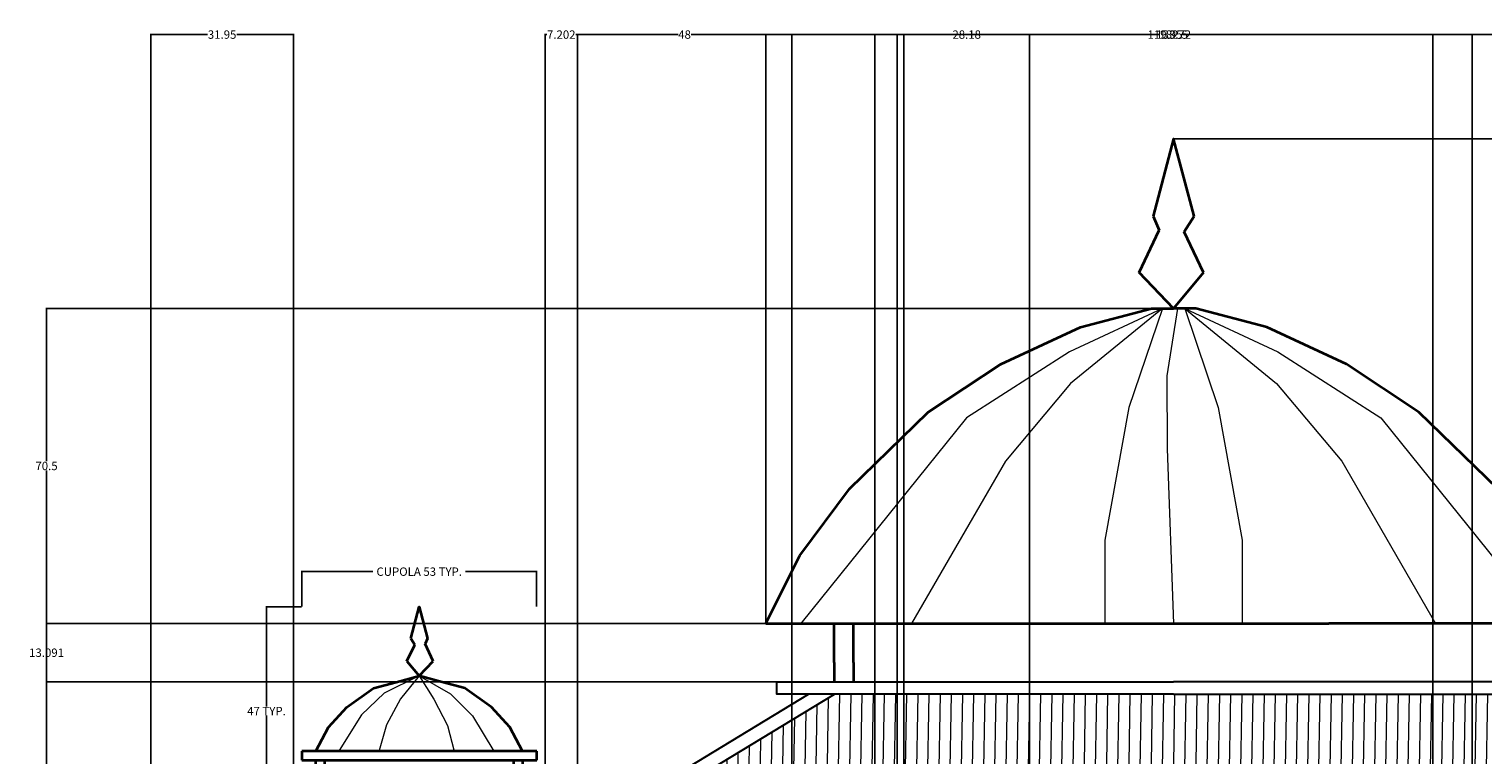
# Model space of a CAD drawing. Units: inches. Extents: x 4 to 523, y 84 to 443.
# Tile 2 of 3: x 4 to 329, y 281 to 443. Entities that reach past the tile are written whole.
import ezdxf

# ---------------------------------------------------------------- set-up
doc = ezdxf.new("R2010")
doc.units = ezdxf.units.IN
doc.header["$MEASUREMENT"] = 0
for name, color, linetype, lineweight in [('A-ANNO-DIMS', 2, 'Continuous', 18), ('A-ROOF', 7, 'Continuous', 30), ('A-ROOF-DETL', 3, 'Continuous', 18), ('A-ROOF-DOME', 7, 'Continuous', 35), ('A-ROOF-PATT', 252, 'Continuous', 13)]:
    doc.layers.add(name, color=color, linetype=linetype, lineweight=lineweight)
doc.styles.get("Standard").update_dxf_attribs({"font": 'arial.ttf'})
doc.dimstyles.get("Standard").update_dxf_attribs({"dimtxt": 1.875, "dimasz": 0.18, "dimexe": 0.18, "dimexo": 0.0625, "dimgap": 0.09, "dimtad": 0, "dimtih": 1, "dimtoh": 1, "dimdec": 4, "dimzin": 0, "dimdsep": 46, "dimlunit": 4, "dimtxsty": 'Standard', "dimcen": 0.09, "dimadec": 0, "dimazin": 0, "dimtfac": 1, "dimtdec": 4, "dimtofl": 0, "dimtmove": 0, "dimatfit": 3, "dimfxl": 1, "dimtolj": 1, "dimtzin": 0, "dimarcsym": 0})

# ---------------------------------------------------------------- blocks, each defined once
blk = doc.blocks.new('CUPOLA-PROFILE')
for p, q in [((52.59, 14.33), (0, 14.33)), ((0, 14.33), (0, 12.33)), ((52.59, 12.33), (52.59, 14.33)), ((0, 12.33), (52.59, 12.33)), ((3.17, 3.77), (3.17, 12.33)), ((5.17, 3.77), (5.17, 12.33)), ((47.49, 3.77), (47.49, 12.33)), ((49.49, 3.77), (49.49, 12.33)), ((3.17, 3.77), (3.17, 0)), ((5.17, 3.77), (5.17, 0)), ((47.49, 3.77), (47.49, 0)), ((49.49, 3.77), (49.49, 0))]:
    blk.add_line(p, q)
for points in [[(24.44, 39.59), (26.29, 46.64), (28.15, 39.59)], [(25.33, 38.18), (24.44, 39.59)], [(28.15, 39.59), (27.62, 38.34)], [(23.56, 34.47), (25.33, 38.18)], [(29.42, 34.47), (27.62, 38.34)], [(23.56, 34.47), (26.29, 31.2)], [(26.29, 31.2), (29.42, 34.47)], [(3.17, 14.33), (6, 19.75), (10.13, 24.22), (16.05, 28.42), (21.12, 29.8), (26.29, 31.2)], [(49.42, 14.33), (46.59, 19.75), (42.46, 24.22), (36.53, 28.42), (31.46, 29.8), (26.29, 31.2)]]:
    blk.add_lwpolyline(points)
blk = doc.blocks.new('*D11')
at = {"layer": 'A-ANNO-DIMS', "color": 0, "lineweight": -2, "transparency": 16777216}
for p, q in [((64.71, 313.84), (64.71, 321.84)), ((64.89, 321.66), (80.62, 321.66)), ((117.12, 321.66), (101.4, 321.66)), ((117.3, 313.84), (117.3, 321.84))]:
    blk.add_line(p, q, dxfattribs=at)
at = {"layer": 'A-ANNO-DIMS', "color": 0, "transparency": 16777216}
for points in [[(64.89, 321.69), (64.89, 321.63), (64.71, 321.66)], [(117.12, 321.69), (117.12, 321.63), (117.3, 321.66)]]:
    blk.add_solid(points, dxfattribs=at)
at = {"layer": 'Defpoints', "color": 0, "transparency": 16777216}
for p in [(117.3, 321.66), (64.71, 313.78), (117.3, 313.78)]:
    blk.add_point(p, dxfattribs=at)
at = {"layer": 'A-ANNO-DIMS', "color": 0, "transparency": 16777216, "insert": (91.01, 321.66), "char_height": 1.875, "attachment_point": 5}
blk.add_mtext('\\A1;CUPOLA 53 TYP.', dxfattribs=at)
blk = doc.blocks.new('*D12')
at = {"layer": 'A-ANNO-DIMS', "color": 0, "lineweight": -2, "transparency": 16777216}
for p, q in [((64.65, 313.78), (56.65, 313.78)), ((56.83, 313.6), (56.83, 291.48)), ((56.83, 267.31), (56.83, 289.43)), ((64.65, 267.13), (56.65, 267.13))]:
    blk.add_line(p, q, dxfattribs=at)
at = {"layer": 'A-ANNO-DIMS', "color": 0, "transparency": 16777216}
for points in [[(56.8, 313.6), (56.86, 313.6), (56.83, 313.78)], [(56.8, 267.31), (56.86, 267.31), (56.83, 267.13)]]:
    blk.add_solid(points, dxfattribs=at)
at = {"layer": 'Defpoints', "color": 0, "transparency": 16777216}
for p in [(56.83, 313.78), (64.71, 313.78), (64.71, 267.13)]:
    blk.add_point(p, dxfattribs=at)
at = {"layer": 'A-ANNO-DIMS', "color": 0, "transparency": 16777216, "insert": (56.83, 290.45), "char_height": 1.875, "attachment_point": 5}
blk.add_mtext('\\A1;47 TYP.', dxfattribs=at)
blk = doc.blocks.new('*D20')
at = {"layer": 'A-ANNO-DIMS', "color": 0, "lineweight": -2, "transparency": 16777216}
for p, q in [((259.93, 418.56), (519, 418.56)), ((518.82, 418.38), (518.82, 265.56)), ((518.82, 110.64), (518.82, 263.46)), ((495.56, 110.46), (519, 110.46))]:
    blk.add_line(p, q, dxfattribs=at)
at = {"layer": 'A-ANNO-DIMS', "color": 0, "transparency": 16777216}
for points in [[(518.79, 418.38), (518.85, 418.38), (518.82, 418.56)], [(518.79, 110.64), (518.85, 110.64), (518.82, 110.46)]]:
    blk.add_solid(points, dxfattribs=at)
at = {"layer": 'Defpoints', "color": 0, "transparency": 16777216}
for p in [(259.87, 418.56), (518.82, 418.56), (495.5, 110.46)]:
    blk.add_point(p, dxfattribs=at)
at = {"layer": 'A-ANNO-DIMS', "color": 0, "transparency": 16777216, "insert": (518.82, 264.51), "char_height": 1.875, "attachment_point": 5}
blk.add_mtext('\\A1;308.1', dxfattribs=at)
blk = doc.blocks.new('*D21')
at = {"layer": 'A-ANNO-DIMS', "color": 0, "lineweight": -2, "transparency": 16777216}
for p, q in [((30.92, 119.64), (30.92, 442.06)), ((31.1, 441.88), (43.64, 441.88)), ((62.69, 441.88), (50.16, 441.88)), ((62.87, 128.52), (62.87, 442.06))]:
    blk.add_line(p, q, dxfattribs=at)
at = {"layer": 'A-ANNO-DIMS', "color": 0, "transparency": 16777216}
for points in [[(31.1, 441.91), (31.1, 441.85), (30.92, 441.88)], [(62.69, 441.91), (62.69, 441.85), (62.87, 441.88)]]:
    blk.add_solid(points, dxfattribs=at)
at = {"layer": 'Defpoints', "color": 0, "transparency": 16777216}
for p in [(62.87, 441.88), (62.87, 128.46), (30.92, 119.58)]:
    blk.add_point(p, dxfattribs=at)
at = {"layer": 'A-ANNO-DIMS', "color": 0, "transparency": 16777216, "insert": (46.9, 441.88), "char_height": 1.875, "attachment_point": 5}
blk.add_mtext('\\A1;31.95', dxfattribs=at)
blk = doc.blocks.new('*D24')
at = {"layer": 'A-ANNO-DIMS', "color": 0, "lineweight": -2, "transparency": 16777216}
for p, q in [((168.55, 310.07), (7.42, 310.07)), ((7.6, 309.89), (7.6, 220.31)), ((7.6, 128.64), (7.6, 218.22)), ((47.09, 128.46), (7.42, 128.46))]:
    blk.add_line(p, q, dxfattribs=at)
at = {"layer": 'A-ANNO-DIMS', "color": 0, "transparency": 16777216}
for points in [[(7.57, 309.89), (7.63, 309.89), (7.6, 310.07)], [(7.57, 128.64), (7.63, 128.64), (7.6, 128.46)]]:
    blk.add_solid(points, dxfattribs=at)
at = {"layer": 'Defpoints', "color": 0, "transparency": 16777216}
for p in [(7.6, 310.07), (168.61, 310.07), (47.15, 128.46)]:
    blk.add_point(p, dxfattribs=at)
at = {"layer": 'A-ANNO-DIMS', "color": 0, "transparency": 16777216, "insert": (7.6, 219.27), "char_height": 1.875, "attachment_point": 5}
blk.add_mtext('\\A1;181.6', dxfattribs=at)
blk = doc.blocks.new('*D25')
at = {"layer": 'A-ANNO-DIMS', "color": 0, "lineweight": -2, "transparency": 16777216}
for p, q in [((168.61, 310.13), (168.61, 442.06)), ((168.79, 441.88), (256.7, 441.88)), ((350.95, 441.88), (263.04, 441.88)), ((351.13, 310.13), (351.13, 442.06))]:
    blk.add_line(p, q, dxfattribs=at)
at = {"layer": 'A-ANNO-DIMS', "color": 0, "transparency": 16777216}
for points in [[(168.79, 441.91), (168.79, 441.85), (168.61, 441.88)], [(350.95, 441.91), (350.95, 441.85), (351.13, 441.88)]]:
    blk.add_solid(points, dxfattribs=at)
at = {"layer": 'Defpoints', "color": 0, "transparency": 16777216}
for p in [(351.13, 441.88), (168.61, 310.07), (351.13, 310.07)]:
    blk.add_point(p, dxfattribs=at)
at = {"layer": 'A-ANNO-DIMS', "color": 0, "transparency": 16777216, "insert": (259.87, 441.88), "char_height": 1.875, "attachment_point": 5}
blk.add_mtext('\\A1;182.5', dxfattribs=at)
blk = doc.blocks.new('*D26')
at = {"layer": 'A-ANNO-DIMS', "color": 0, "lineweight": -2, "transparency": 16777216}
for p, q in [((254.84, 380.57), (7.42, 380.57)), ((7.6, 380.39), (7.6, 346.37)), ((7.6, 310.25), (7.6, 344.27)), ((168.55, 310.07), (7.42, 310.07))]:
    blk.add_line(p, q, dxfattribs=at)
at = {"layer": 'A-ANNO-DIMS', "color": 0, "transparency": 16777216}
for points in [[(7.57, 380.39), (7.63, 380.39), (7.6, 380.57)], [(7.57, 310.25), (7.63, 310.25), (7.6, 310.07)]]:
    blk.add_solid(points, dxfattribs=at)
at = {"layer": 'Defpoints', "color": 0, "transparency": 16777216}
for p in [(7.6, 380.57), (254.9, 380.57), (168.61, 310.07)]:
    blk.add_point(p, dxfattribs=at)
at = {"layer": 'A-ANNO-DIMS', "color": 0, "transparency": 16777216, "insert": (7.6, 345.32), "char_height": 1.875, "attachment_point": 5}
blk.add_mtext('\\A1;70.5', dxfattribs=at)
blk = doc.blocks.new('*D27')
at = {"layer": 'A-ANNO-DIMS', "color": 0, "lineweight": -2, "transparency": 16777216}
for p, q in [((168.55, 310.07), (7.42, 310.07)), ((7.6, 309.89), (7.6, 304.57)), ((7.6, 297.16), (7.6, 302.48)), ((170.97, 296.98), (7.42, 296.98))]:
    blk.add_line(p, q, dxfattribs=at)
at = {"layer": 'A-ANNO-DIMS', "color": 0, "transparency": 16777216}
for points in [[(7.57, 309.89), (7.63, 309.89), (7.6, 310.07)], [(7.57, 297.16), (7.63, 297.16), (7.6, 296.98)]]:
    blk.add_solid(points, dxfattribs=at)
at = {"layer": 'Defpoints', "color": 0, "transparency": 16777216}
for p in [(168.61, 310.07), (7.6, 296.98), (171.03, 296.98)]:
    blk.add_point(p, dxfattribs=at)
at = {"layer": 'A-ANNO-DIMS', "color": 0, "transparency": 16777216, "insert": (7.6, 303.52), "char_height": 1.875, "attachment_point": 5}
blk.add_mtext('\\A1;13.091', dxfattribs=at)
blk = doc.blocks.new('*D28')
at = {"layer": 'A-ANNO-DIMS', "color": 0, "lineweight": -2, "transparency": 16777216}
for p, q in [((193.01, 215.71), (193.01, 442.06)), ((193.19, 441.88), (255.99, 441.88)), ((326.55, 441.88), (263.75, 441.88)), ((326.73, 215.71), (326.73, 442.06))]:
    blk.add_line(p, q, dxfattribs=at)
at = {"layer": 'A-ANNO-DIMS', "color": 0, "transparency": 16777216}
for points in [[(193.19, 441.91), (193.19, 441.85), (193.01, 441.88)], [(326.55, 441.91), (326.55, 441.85), (326.73, 441.88)]]:
    blk.add_solid(points, dxfattribs=at)
at = {"layer": 'Defpoints', "color": 0, "transparency": 16777216}
for p in [(326.73, 441.88), (193.01, 215.64), (326.73, 215.64)]:
    blk.add_point(p, dxfattribs=at)
at = {"layer": 'A-ANNO-DIMS', "color": 0, "transparency": 16777216, "insert": (259.87, 441.88), "char_height": 1.875, "attachment_point": 5}
blk.add_mtext('\\A1;133.72', dxfattribs=at)
blk = doc.blocks.new('*D30')
at = {"layer": 'A-ANNO-DIMS', "color": 0, "lineweight": -2, "transparency": 16777216}
for p, q in [((126.41, 193.37), (126.41, 442.06)), ((126.59, 441.88), (148.94, 441.88)), ((174.23, 441.88), (151.88, 441.88)), ((174.41, 193.37), (174.41, 442.06))]:
    blk.add_line(p, q, dxfattribs=at)
at = {"layer": 'A-ANNO-DIMS', "color": 0, "transparency": 16777216}
for points in [[(126.59, 441.91), (126.59, 441.85), (126.41, 441.88)], [(174.23, 441.91), (174.23, 441.85), (174.41, 441.88)]]:
    blk.add_solid(points, dxfattribs=at)
at = {"layer": 'Defpoints', "color": 0, "transparency": 16777216}
for p in [(174.41, 441.88), (126.41, 193.3), (174.41, 193.3)]:
    blk.add_point(p, dxfattribs=at)
at = {"layer": 'A-ANNO-DIMS', "color": 0, "transparency": 16777216, "insert": (150.41, 441.88), "char_height": 1.875, "attachment_point": 5}
blk.add_mtext('\\A1;48', dxfattribs=at)
blk = doc.blocks.new('*D32')
at = {"layer": 'A-ANNO-DIMS', "color": 0, "lineweight": -2, "transparency": 16777216}
for p, q in [((197.96, 203.64), (197.96, 442.06)), ((198.14, 441.88), (254.04, 441.88)), ((317.74, 441.88), (261.84, 441.88)), ((317.92, 203.64), (317.92, 442.06))]:
    blk.add_line(p, q, dxfattribs=at)
at = {"layer": 'A-ANNO-DIMS', "color": 0, "transparency": 16777216}
for points in [[(198.14, 441.91), (198.14, 441.85), (197.96, 441.88)], [(317.74, 441.91), (317.74, 441.85), (317.92, 441.88)]]:
    blk.add_solid(points, dxfattribs=at)
at = {"layer": 'Defpoints', "color": 0, "transparency": 16777216}
for p in [(317.92, 441.88), (197.96, 203.58), (317.92, 203.58)]:
    blk.add_point(p, dxfattribs=at)
at = {"layer": 'A-ANNO-DIMS', "color": 0, "transparency": 16777216, "insert": (257.94, 441.88), "char_height": 1.875, "attachment_point": 5}
blk.add_mtext('\\A1;119.95', dxfattribs=at)
blk = doc.blocks.new('*D36')
at = {"layer": 'A-ANNO-DIMS', "color": 0, "lineweight": -2, "transparency": 16777216}
for p, q in [((119.21, 120.55), (119.21, 442.06)), ((119.39, 441.88), (119.57, 441.88)), ((126.23, 441.88), (126.05, 441.88)), ((126.41, 133.37), (126.41, 442.06))]:
    blk.add_line(p, q, dxfattribs=at)
at = {"layer": 'A-ANNO-DIMS', "color": 0, "transparency": 16777216}
for points in [[(119.39, 441.91), (119.39, 441.85), (119.21, 441.88)], [(126.23, 441.91), (126.23, 441.85), (126.41, 441.88)]]:
    blk.add_solid(points, dxfattribs=at)
at = {"layer": 'Defpoints', "color": 0, "transparency": 16777216}
for p in [(126.41, 441.88), (126.41, 133.3), (119.21, 120.48)]:
    blk.add_point(p, dxfattribs=at)
at = {"layer": 'A-ANNO-DIMS', "color": 0, "transparency": 16777216, "insert": (122.81, 441.88), "char_height": 1.875, "attachment_point": 5}
blk.add_mtext('\\A1;7.202', dxfattribs=at)
blk = doc.blocks.new('*D39')
at = {"layer": 'A-ANNO-DIMS', "color": 0, "lineweight": -2, "transparency": 16777216}
for p, q in [((199.46, 193.37), (199.46, 442.06)), ((199.64, 441.88), (210.28, 441.88)), ((227.46, 441.88), (216.82, 441.88)), ((227.64, 193.37), (227.64, 442.06))]:
    blk.add_line(p, q, dxfattribs=at)
at = {"layer": 'A-ANNO-DIMS', "color": 0, "transparency": 16777216}
for points in [[(199.64, 441.91), (199.64, 441.85), (199.46, 441.88)], [(227.46, 441.91), (227.46, 441.85), (227.64, 441.88)]]:
    blk.add_solid(points, dxfattribs=at)
at = {"layer": 'Defpoints', "color": 0, "transparency": 16777216}
for p in [(227.64, 441.88), (199.46, 193.3), (227.64, 193.3)]:
    blk.add_point(p, dxfattribs=at)
at = {"layer": 'A-ANNO-DIMS', "color": 0, "transparency": 16777216, "insert": (213.55, 441.88), "char_height": 1.875, "attachment_point": 5}
blk.add_mtext('\\A1;28.18', dxfattribs=at)

msp = doc.modelspace()

# ---------------------------------------------------------------- hatches: boundary and pattern name
at = {"layer": 'A-ROOF-PATT'}
h = msp.add_hatch(dxfattribs=at)
h.set_pattern_fill('ANSI31', color=256, scale=20, angle=44)
h.paths.add_polyline_path([(335.7846, 294.2465), (329.6848, 294.2465), (259.8699, 294.2465), (190.0549, 294.2465), (183.9551, 294.2465), (119.2078, 254.9874), (185.0083, 254.9874), (185.0083, 259.3969), (185.0083, 268.2159), (179.3813, 268.2159), (179.3813, 270.5155), (240.8614, 270.5155), (259.8699, 270.5155), (278.8783, 270.5155), (340.3584, 270.5155), (340.3584, 268.2159), (334.7314, 268.2159), (334.7314, 259.3969), (334.7314, 254.9874), (400.5319, 254.9874)])

# ---------------------------------------------------------------- linework, layer by layer
at = {"layer": 'A-ROOF'}
for p, q in [((119.2078, 254.9874), (183.9551, 294.2465)), ((119.2078, 258.4958), (178.169, 294.2465))]:
    msp.add_line(p, q, dxfattribs=at)
for points in [[(259.8699, 294.2465), (190.0549, 294.2465), (171.0286, 294.2465), (171.0286, 296.9786), (259.8699, 296.9786)], [(259.8699, 294.2465), (329.6848, 294.2465), (348.7111, 294.2465), (348.7111, 296.9786), (259.8699, 296.9786)]]:
    msp.add_lwpolyline(points, dxfattribs=at)
at = {"layer": 'A-ROOF-DETL'}
for p, q in [((73.1151, 281.6072), (73.025, 281.4574)), ((82.0403, 281.6072), (81.9972, 281.4574))]:
    msp.add_line(p, q, dxfattribs=at)
for points in [[(257.3839, 380.5683), (236.5791, 370.8672), (213.5203, 356.0749), (176.4022, 310.0699)], [(257.3839, 380.5683), (236.815, 363.7483), (222.2238, 346.3552), (201.2329, 310.0699)], [(257.3839, 380.5683), (249.8704, 358.3769), (244.4946, 328.7063), (244.4946, 310.0699)], [(260.7414, 380.5683), (258.3853, 365.5308), (258.4598, 349.1416), (259.8699, 310.0699)], [(262.3558, 380.5683), (283.1606, 370.8672), (306.2195, 356.0749), (343.3375, 310.0699)], [(262.3558, 380.5683), (282.9247, 363.7483), (297.5159, 346.3552), (318.5068, 310.0699)], [(262.3558, 380.5683), (269.8693, 358.3769), (275.2451, 328.7063), (275.2451, 310.0699)], [(91.0136, 298.3231), (83.1473, 294.426), (78.0966, 289.5867), (73.1151, 281.6072)], [(91.0136, 298.3231), (86.8143, 293.1816), (83.7008, 287.3744), (82.0403, 281.6072)], [(91.0136, 298.3231), (97.9897, 294.2948), (102.9541, 289.367), (107.6998, 281.4574)], [(91.0136, 298.3231), (94.3013, 293.1154), (97.3116, 287.2542), (98.87, 281.4585)]]:
    msp.add_lwpolyline(points, dxfattribs=at)
at = {"layer": 'A-ROOF-DOME'}
for p, q in [((168.6117, 310.0699), (225.1561, 310.0699)), ((183.8664, 301.3423), (183.8664, 310.0699)), ((188.2508, 301.3423), (188.2508, 310.0699)), ((225.1561, 310.0699), (294.5837, 310.0699)), ((352.2366, 310.0699), (294.5837, 310.0699)), ((183.8664, 301.3423), (183.8664, 296.9786)), ((188.2508, 301.3423), (188.2508, 296.9786))]:
    msp.add_line(p, q, dxfattribs=at)
for points in [[(264.4378, 401.218), (259.8702, 418.5576), (255.3026, 401.218)], [(255.3026, 401.218), (256.6076, 398.1306)], [(262.2461, 397.7514), (264.4378, 401.218)], [(252.1846, 388.6082), (256.6076, 398.1306)], [(266.5944, 388.6082), (262.2461, 397.7514)], [(259.8699, 380.5683), (252.1846, 388.6082)], [(266.5944, 388.6082), (259.8699, 380.5683)], [(168.6117, 310.0699), (176.2081, 325.3117), (187.3079, 340.1657), (204.9487, 357.3962), (221.202, 368.091), (239.041, 376.4092), (254.8979, 380.5683), (259.8699, 380.5683)], [(351.128, 310.0699), (343.5316, 325.3117), (332.4318, 340.1657), (314.791, 357.3962), (298.5377, 368.091), (280.6987, 376.4092), (264.8418, 380.5683), (259.8699, 380.5683)]]:
    msp.add_lwpolyline(points, dxfattribs=at)

# ---------------------------------------------------------------- block references
msp.add_blockref('CUPOLA-PROFILE', (64.714, 267.131), dxfattribs=at)

# ---------------------------------------------------------------- dimensions: what is measured, and where the dimension line sits
at = {"layer": 'A-ANNO-DIMS'}
for base, p1, p2, override, picture, middle in [((62.873, 441.8826), (30.9213, 119.5803), (62.873, 128.4611), {"dimdec": 2, "dimlfac": 1, "dimrnd": 0, "dimzin": 0, "dimdsep": 46, "dimlunit": 2}, '*D21', (46.8972, 441.8826)), ((126.4097, 441.8826), (119.2078, 120.483), (126.4097, 133.3038), {"dimdec": 3, "dimlfac": 1, "dimrnd": 0, "dimzin": 0, "dimdsep": 46, "dimlunit": 2}, '*D36', (122.8087, 441.8826)), ((174.4097, 441.8826), (126.4097, 193.3038), (174.4097, 193.3038), {"dimdec": 0, "dimlfac": 1, "dimrnd": 0, "dimzin": 0, "dimdsep": 46, "dimlunit": 2}, '*D30', (150.4097, 441.8826)), ((351.128, 441.8826), (168.6117, 310.0699), (351.128, 310.0699), {"dimdec": 1, "dimlfac": 1, "dimrnd": 0, "dimzin": 0, "dimdsep": 46, "dimlunit": 2}, '*D25', (259.8699, 441.8826)), ((326.7314, 441.8826), (193.0083, 215.6431), (326.7314, 215.6431), {"dimdec": 2, "dimlfac": 1, "dimrnd": 0, "dimzin": 0, "dimdsep": 46, "dimlunit": 2}, '*D28', (259.8699, 441.8826)), ((317.9162, 441.8826), (197.9616, 203.5817), (317.9162, 203.5817), {"dimdec": 2, "dimlfac": 1, "dimrnd": 0, "dimzin": 0, "dimdsep": 46, "dimlunit": 2}, '*D32', (257.9389, 441.8826)), ((227.6434, 441.8826), (199.4616, 193.3038), (227.6434, 193.3038), {"dimdec": 2, "dimlfac": 1, "dimrnd": 0, "dimzin": 0, "dimdsep": 46, "dimlunit": 2}, '*D39', (213.5525, 441.8826))]:
    dim = msp.add_linear_dim(base=base, p1=p1, p2=p2, dimstyle='Standard', override=override, dxfattribs=at)
    dim.commit()
    dim.dimension.update_dxf_attribs({"geometry": picture, "text_midpoint": middle})
for base, p1, p2, override, picture, middle in [((518.8204, 418.5576), (495.4954, 110.4611), (259.8702, 418.5576), {"dimdec": 1, "dimlfac": 1, "dimrnd": 0, "dimzin": 0, "dimdsep": 46, "dimlunit": 2}, '*D20', (518.8204, 264.5094)), ((7.5963, 380.5683), (168.6117, 310.0699), (254.8979, 380.5683), {"dimdec": 1, "dimlfac": 1, "dimrnd": 0, "dimzin": 0, "dimdsep": 46, "dimlunit": 2}, '*D26', (7.5963, 345.3191)), ((7.5963, 296.9786), (168.6117, 310.0699), (171.0286, 296.9786), {"dimdec": 3, "dimlfac": 1, "dimrnd": 0, "dimzin": 0, "dimdsep": 46, "dimlunit": 2}, '*D27', (7.5963, 303.5242)), ((7.5963, 310.0699), (47.1512, 128.4611), (168.6117, 310.0699), {"dimdec": 1, "dimlfac": 1, "dimrnd": 0, "dimzin": 0, "dimdsep": 46, "dimlunit": 2}, '*D24', (7.5963, 219.2655))]:
    dim = msp.add_linear_dim(base=base, p1=p1, p2=p2, angle=90, dimstyle='Standard', override=override, dxfattribs=at)
    dim.commit()
    dim.dimension.update_dxf_attribs({"geometry": picture, "text_midpoint": middle})
dim = msp.add_linear_dim(base=(117.3028, 321.6641), p1=(64.7144, 313.7758), p2=(117.3028, 313.7758), text='CUPOLA <> TYP.', dimstyle='Standard', override={"dimdec": 0, "dimlfac": 1, "dimrnd": 0, "dimzin": 0, "dimdsep": 46, "dimlunit": 2}, dxfattribs=at)
dim.commit()
dim.dimension.update_dxf_attribs({"geometry": '*D11', "text_midpoint": (91.0086, 321.6641)})
dim = msp.add_linear_dim(base=(56.8261, 313.7758), p1=(64.7144, 267.1306), p2=(64.7144, 313.7758), angle=90, text='<> TYP.', dimstyle='Standard', override={"dimdec": 0, "dimlfac": 1, "dimrnd": 0, "dimzin": 0, "dimdsep": 46, "dimlunit": 2}, dxfattribs=at)
dim.commit()
dim.dimension.update_dxf_attribs({"geometry": '*D12', "text_midpoint": (56.8261, 290.4532)})

doc.saveas('drawing.dxf')
